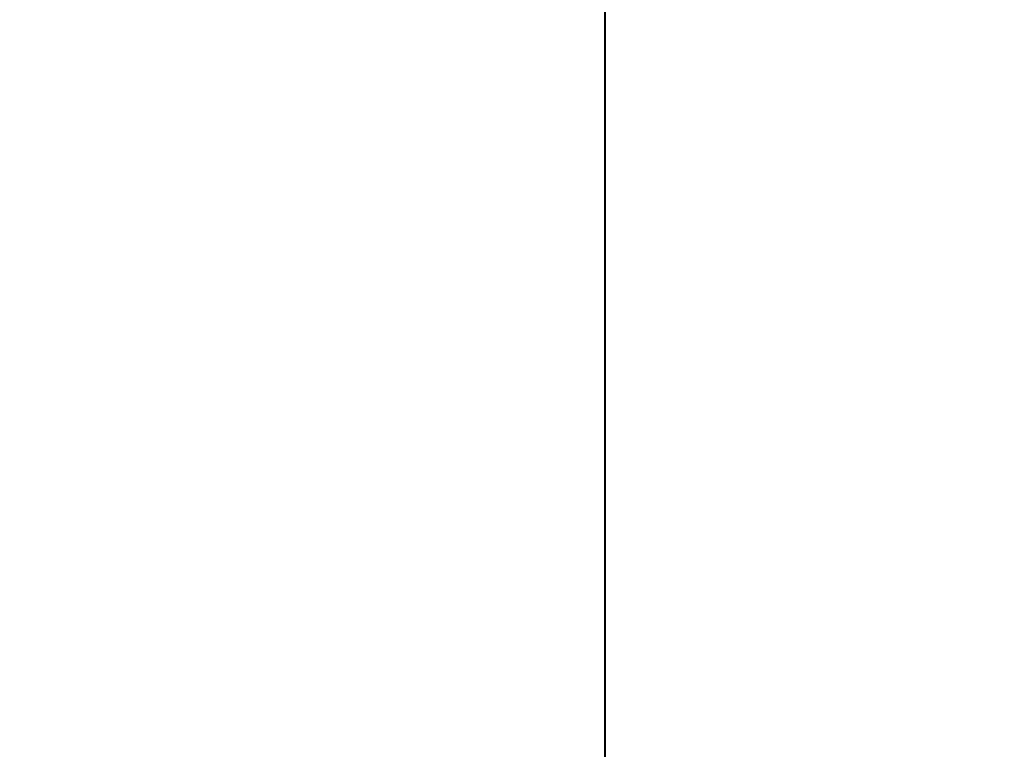
# Model space of a CAD drawing. Units: inches. Extents: x 459864 to 460310, y 324185 to 324787.
# Tile 86 of 112: x 460247.1043 to 460247.12218, y 324283.49543 to 324283.50868. Entities that reach past the tile are written whole.
import ezdxf

# ---------------------------------------------------------------- set-up
doc = ezdxf.new("R2010")
doc.units = ezdxf.units.IN
doc.layers.add('A-ANNO-DIMS', color=2, linetype='Continuous', lineweight=18)
doc.layers.add('A-WALL', color=7, linetype='Continuous', lineweight=40)
doc.styles.get("Standard").update_dxf_attribs({"font": 'arial.ttf'})
doc.dimstyles.new('ISO-25', dxfattribs={"dimtxt": 6, "dimasz": 2.5, "dimexe": 1.25, "dimexo": 0.625, "dimtad": 1, "dimdec": 1, "dimlunit": 3, "dimtxsty": 'Standard', "dimcen": 2.5, "dimadec": 0, "dimazin": 0, "dimtfac": 1, "dimtdec": 1, "dimtmove": 0, "dimatfit": 3, "dimfxl": 1, "dimarcsym": 0})

# ---------------------------------------------------------------- blocks, each defined once
blk = doc.blocks.new('*D21')
at = {"layer": 'A-ANNO-DIMS', "color": 0, "lineweight": -2, "transparency": 16777216}
for p, q in [((460247.739927, 324715.483233), (460309.580369, 324715.483233)), ((460308.330369, 324712.983233), (460308.330369, 324285.983233)), ((460247.739927, 324283.483233), (460309.580369, 324283.483233))]:
    blk.add_line(p, q, dxfattribs=at)
at = {"layer": 'A-ANNO-DIMS', "color": 0, "transparency": 16777216}
for points in [[(460307.913702, 324712.983233), (460308.747035, 324712.983233), (460308.330369, 324715.483233)], [(460307.913702, 324285.983233), (460308.747035, 324285.983233), (460308.330369, 324283.483233)]]:
    blk.add_solid(points, dxfattribs=at)
at = {"layer": 'Defpoints', "color": 0, "transparency": 16777216}
for p in [(460247.114927, 324715.483233), (460247.114927, 324283.483233), (460308.330369, 324283.483233)]:
    blk.add_point(p, dxfattribs=at)
at = {"layer": 'A-ANNO-DIMS', "color": 0, "transparency": 16777216, "insert": (460304.639884, 324499.483233), "char_height": 6, "attachment_point": 5, "rotation": 90}
blk.add_mtext("36'", dxfattribs=at)
blk = doc.blocks.new('*D62')
at = {"layer": 'A-ANNO-DIMS', "color": 0, "lineweight": -2, "transparency": 16777216}
for p, q in [((460247.739927, 324332.73872), (460278.764927, 324332.73872)), ((460277.514927, 324330.23872), (460277.514927, 324285.983233)), ((460247.739927, 324283.483233), (460278.764927, 324283.483233))]:
    blk.add_line(p, q, dxfattribs=at)
at = {"layer": 'A-ANNO-DIMS', "color": 0, "transparency": 16777216}
for points in [[(460277.09826, 324330.23872), (460277.931594, 324330.23872), (460277.514927, 324332.73872)], [(460277.09826, 324285.983233), (460277.931594, 324285.983233), (460277.514927, 324283.483233)]]:
    blk.add_solid(points, dxfattribs=at)
at = {"layer": 'Defpoints', "color": 0, "transparency": 16777216}
for p in [(460247.114927, 324332.73872), (460247.114927, 324283.483233), (460277.514927, 324283.483233)]:
    blk.add_point(p, dxfattribs=at)
at = {"layer": 'A-ANNO-DIMS', "color": 0, "transparency": 16777216, "insert": (460273.787608, 324308.110976), "char_height": 6, "attachment_point": 5, "rotation": 90}
blk.add_mtext('4\'-1 1/2"', dxfattribs=at)
blk = doc.blocks.new('*D67')
at = {"layer": 'A-ANNO-DIMS', "color": 0, "lineweight": -2, "transparency": 16777216}
for p, q in [((460208.114927, 324284.108233), (460208.114927, 324315.133233)), ((460247.114927, 324284.108233), (460247.114927, 324315.133233)), ((460210.614927, 324313.883233), (460244.614927, 324313.883233))]:
    blk.add_line(p, q, dxfattribs=at)
at = {"layer": 'A-ANNO-DIMS', "color": 0, "transparency": 16777216}
for points in [[(460210.614927, 324314.2999), (460210.614927, 324313.466566), (460208.114927, 324313.883233)], [(460244.614927, 324314.2999), (460244.614927, 324313.466566), (460247.114927, 324313.883233)]]:
    blk.add_solid(points, dxfattribs=at)
at = {"layer": 'Defpoints', "color": 0, "transparency": 16777216}
for p in [(460247.114927, 324313.883233), (460208.114927, 324283.483233), (460247.114927, 324283.483233)]:
    blk.add_point(p, dxfattribs=at)
at = {"layer": 'A-ANNO-DIMS', "color": 0, "transparency": 16777216, "insert": (460227.614927, 324317.573717), "char_height": 6, "attachment_point": 5}
blk.add_mtext('3\'-3"', dxfattribs=at)

msp = doc.modelspace()

# ---------------------------------------------------------------- linework, layer by layer
at = {"layer": 'A-WALL'}
msp.add_line((460247.114927, 324470.983233), (460247.114927, 324283.483233), dxfattribs=at)

# ---------------------------------------------------------------- dimensions: what is measured, and where the dimension line sits
at = {"layer": 'A-ANNO-DIMS'}
for base, p1, angle, override, picture, middle in [((460308.330369, 324283.483233), (460247.114927, 324715.483233), 90, {"dimclrd": 0, "dimclre": 0, "dimclrt": 0}, '*D21', (460304.639884, 324499.483233)), ((460277.514927, 324283.483233), (460247.114927, 324332.73872), 270, {"dimdec": 1, "dimlfac": 1, "dimrnd": 0, "dimzin": 1, "dimdsep": 46, "dimlunit": 4, "dimfrac": 2}, '*D62', (460273.787608, 324308.110976))]:
    dim = msp.add_linear_dim(base=base, p1=p1, p2=(460247.114927, 324283.483233), angle=angle, dimstyle='ISO-25', override=override, dxfattribs=at)
    dim.commit()
    dim.dimension.update_dxf_attribs({"geometry": picture, "text_midpoint": middle})
dim = msp.add_linear_dim(base=(460247.114927, 324313.883233), p1=(460208.114927, 324283.483233), p2=(460247.114927, 324283.483233), dimstyle='ISO-25', override={"dimdec": 1, "dimlfac": 1, "dimrnd": 0, "dimzin": 1, "dimdsep": 46, "dimlunit": 4, "dimfrac": 2}, dxfattribs=at)
dim.commit()
dim.dimension.update_dxf_attribs({"geometry": '*D67', "text_midpoint": (460227.614927, 324317.573717)})

doc.saveas('drawing.dxf')
